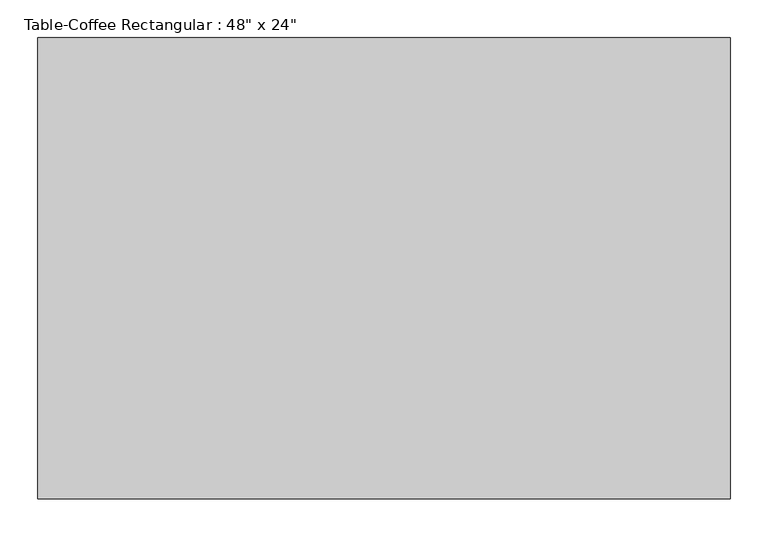
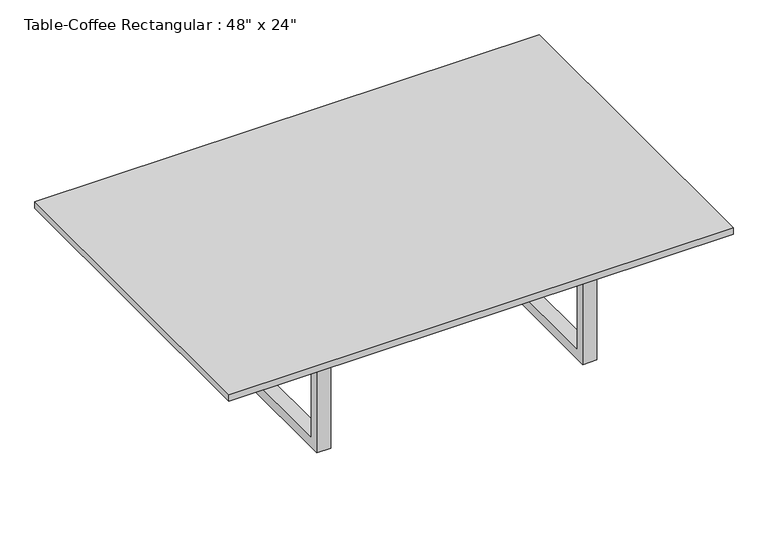
"""IFC4 building model written with IfcOpenShell, lengths in millimetres: furniture geometry."""

from ifc_helpers import new_model, si_unit, frame, origin, place, context, project, spatial, polyline, outline, extrude, source, transform, mapped, element, save


def furniture_e479396c(model_context):
    return source(origin(), model_context, "Body", "SweptSolid", [
        extrude(outline(polyline([(1070.5336303, 674.4108318), (1070.5336303, 64.8108318), (156.1336303, 64.8108318), (156.1336303, 674.4108318), (1070.5336303, 674.4108318)])), frame((0.0, 0.0, 215.9), z_axis=(0.0, 0.0, 1.0), x_axis=(1.0, 0.0, 0.0)), (0.0, 0.0, 1.0), 12.7),
        extrude(outline(polyline([(141.0108318, 215.9), (598.2108318, 215.9), (598.2108318, 0.0), (141.0108318, 0.0), (141.0108318, 215.9)]), holes=[polyline([(160.0608318, 196.85), (160.0608318, 19.05), (579.1608318, 19.05), (579.1608318, 196.85), (160.0608318, 196.85)])]), frame((359.3336303, 0.0, 0.0), z_axis=(1.0, 0.0, 0.0), x_axis=(0.0, 1.0, 0.0)), (0.0, 0.0, 1.0), 25.4),
        extrude(outline(polyline([(141.0108318, 215.9), (598.2108318, 215.9), (598.2108318, 0.0), (141.0108318, 0.0), (141.0108318, 215.9)]), holes=[polyline([(160.0608318, 196.85), (160.0608318, 19.05), (579.1608318, 19.05), (579.1608318, 196.85), (160.0608318, 196.85)])]), frame((841.9336303, 0.0, 0.0), z_axis=(1.0, 0.0, 0.0), x_axis=(0.0, 1.0, 0.0)), (0.0, 0.0, 1.0), 25.4),
        extrude(outline(polyline([(841.9336303, 379.1358318), (841.9336303, 360.0858318), (384.7336303, 360.0858318), (384.7336303, 379.1358318), (841.9336303, 379.1358318)])), frame((0.0, 0.0, 196.85), z_axis=(0.0, 0.0, 1.0), x_axis=(1.0, 0.0, 0.0)), (0.0, 0.0, 1.0), 19.05),
    ])


if __name__ == "__main__":
    model = new_model("IFC4")
    model_context = context("Model", 3, world=origin())
    ifc_project = project(units=[si_unit("LENGTHUNIT", "METRE", prefix="MILLI")], contexts=[model_context])
    site = spatial("IfcSite", under=ifc_project)
    building = spatial("IfcBuilding", under=site)
    placement = place(None, origin())
    furniture_shape = furniture_e479396c(model_context)
    element("IfcFurniture", 1, ObjectType="Table-Coffee Rectangular : 48\" x 24\"", at=placement, inside=building, context=model_context, shape_type="MappedRepresentation", body=[
        mapped(furniture_shape, transform((0.0, 0.0, 0.0), x_axis=(1.0, 0.0, 0.0), y_axis=(0.0, 1.0, 0.0), z_axis=(0.0, 0.0, 1.0))),
    ])
    save(model, "model.ifc")

# Revit data of these elements
# Type "Table-Coffee Rectangular : 48\" x 24\""
#   Assembly Code = "E2020200"
#   Height = 0' - 9"
#   Length = 3' - 0"
#   Width = 2' - 0"
#   Base Material = Metal - Chrome
#   Table Top Material = Laminate - Ivory,Matte
#   Default Elevation = 0
# Element 1 (IfcFurniture, "Table-Coffee Rectangular : 48\" x 24\"")
#   Materials on its faces: "Metal - Chrome", "Laminate - Ivory,Matte"
# Materials
#   "Metal - Chrome": colour RGB 57 57 57, transparency 0
#   "Laminate - Ivory,Matte": colour RGB 127 127 127, transparency 0
